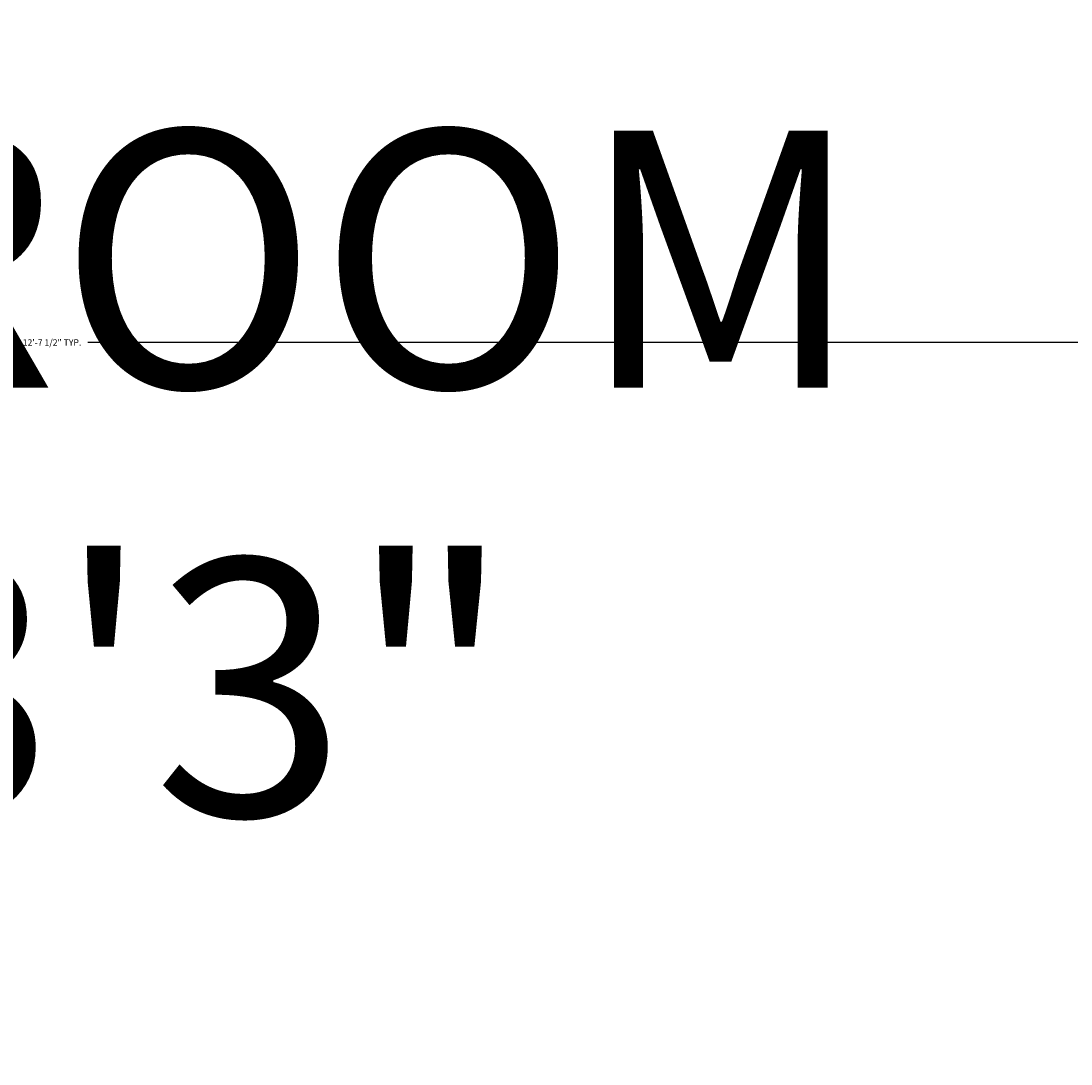
# Model space of a CAD drawing. Units: inches. Extents: x 182 to 1022, y -617 to 111.
# Tile 6 of 33: x 334 to 363, y -340 to -310. Entities that reach past the tile are written whole.
import ezdxf

# ---------------------------------------------------------------- set-up
doc = ezdxf.new("R2010")
doc.units = ezdxf.units.IN
doc.header["$MEASUREMENT"] = 0
doc.layers.add('A-ANNO-DIMS', color=2, linetype='Continuous', lineweight=18)
doc.layers.add('A-AREA-IDEN', color=8, linetype='Continuous', lineweight=18)
doc.styles.get("Standard").update_dxf_attribs({"font": 'arial.ttf'})
doc.dimstyles.get("Standard").update_dxf_attribs({"dimtxt": 0.18, "dimasz": 0.18, "dimexe": 0.18, "dimexo": 0.0625, "dimgap": 0.09, "dimtad": 0, "dimtih": 1, "dimtoh": 1, "dimdec": 1, "dimzin": 0, "dimdsep": 46, "dimlunit": 4, "dimtxsty": 'Standard', "dimcen": 0.09, "dimadec": 0, "dimazin": 0, "dimtfac": 1, "dimtdec": 1, "dimtofl": 0, "dimtmove": 0, "dimatfit": 3, "dimfxl": 1, "dimtolj": 1, "dimtzin": 0, "dimarcsym": 0})

# ---------------------------------------------------------------- blocks, each defined once
blk = doc.blocks.new('*D26')
at = {"layer": 'A-ANNO-DIMS', "color": 0, "lineweight": -2, "transparency": 16777216}
for p, q in [((257.848, -296.884), (257.848, -319.733)), ((409.388, -296.884), (409.388, -319.733)), ((258.028, -319.553), (331.642, -319.553)), ((409.208, -319.553), (335.594, -319.553))]:
    blk.add_line(p, q, dxfattribs=at)
at = {"layer": 'A-ANNO-DIMS', "color": 0, "transparency": 16777216}
for points in [[(258.028, -319.523), (258.028, -319.583), (257.848, -319.553)], [(409.208, -319.523), (409.208, -319.583), (409.388, -319.553)]]:
    blk.add_solid(points, dxfattribs=at)
at = {"layer": 'Defpoints', "color": 0, "transparency": 16777216}
for p in [(257.848, -296.822), (409.388, -296.822), (409.388, -319.553)]:
    blk.add_point(p, dxfattribs=at)
at = {"layer": 'A-ANNO-DIMS', "color": 0, "transparency": 16777216, "insert": (333.618, -319.553), "char_height": 0.18, "attachment_point": 5}
blk.add_mtext('\\A1;LOUNGE GROUP 12\'-7 1/2" TYP.', dxfattribs=at)
blk = doc.blocks.new('*D39')
at = {"layer": 'A-ANNO-DIMS', "color": 0, "lineweight": -2, "transparency": 16777216}
for p, q in [((238.398, -288.54), (1015.285, -288.54)), ((1015.105, -288.72), (1015.105, -346.775)), ((1015.105, -405.193), (1015.105, -347.138)), ((238.427, -405.373), (1015.285, -405.373))]:
    blk.add_line(p, q, dxfattribs=at)
at = {"layer": 'A-ANNO-DIMS', "color": 0, "transparency": 16777216}
for points in [[(1015.075, -288.72), (1015.135, -288.72), (1015.105, -288.54)], [(1015.075, -405.193), (1015.135, -405.193), (1015.105, -405.373)]]:
    blk.add_solid(points, dxfattribs=at)
at = {"layer": 'Defpoints', "color": 0, "transparency": 16777216}
for p in [(238.335, -288.54), (1015.105, -288.54), (238.364, -405.373)]:
    blk.add_point(p, dxfattribs=at)
at = {"layer": 'A-ANNO-DIMS', "color": 0, "transparency": 16777216, "insert": (1015.105, -346.956), "char_height": 0.18, "attachment_point": 5}
blk.add_mtext('\\A1;9\'-9"', dxfattribs=at)

msp = doc.modelspace()

# ---------------------------------------------------------------- texts
at = {"layer": 'A-AREA-IDEN', "insert": (286.446, -313.558), "char_height": 7.27028, "attachment_point": 1}
msp.add_mtext_dynamic_manual_height_columns('    LIVING ROOM\\P        16\'X23\'3"', width=90.78123, gutter_width=1.212, heights=[0], dxfattribs=at)

# ---------------------------------------------------------------- dimensions: what is measured, and where the dimension line sits
at = {"layer": 'A-ANNO-DIMS'}
dim = msp.add_linear_dim(base=(1015.105, -288.54), p1=(238.364, -405.373), p2=(238.335, -288.54), angle=90, dimstyle='Standard', override={"dimdec": 1, "dimlfac": 1, "dimrnd": 0, "dimzin": 1, "dimdsep": 46, "dimlunit": 4, "dimfrac": 2}, dxfattribs=at)
dim.commit()
dim.dimension.update_dxf_attribs({"geometry": '*D39', "text_midpoint": (1015.105, -346.956)})
dim = msp.add_linear_dim(base=(409.388, -319.553), p1=(257.848, -296.822), p2=(409.388, -296.822), text='LOUNGE GROUP <> TYP.', dimstyle='Standard', override={"dimdec": 1, "dimlfac": 1, "dimrnd": 0, "dimzin": 1, "dimdsep": 46, "dimlunit": 4, "dimfrac": 2}, dxfattribs=at)
dim.commit()
dim.dimension.update_dxf_attribs({"geometry": '*D26', "text_midpoint": (333.618, -319.553)})

doc.saveas('drawing.dxf')
